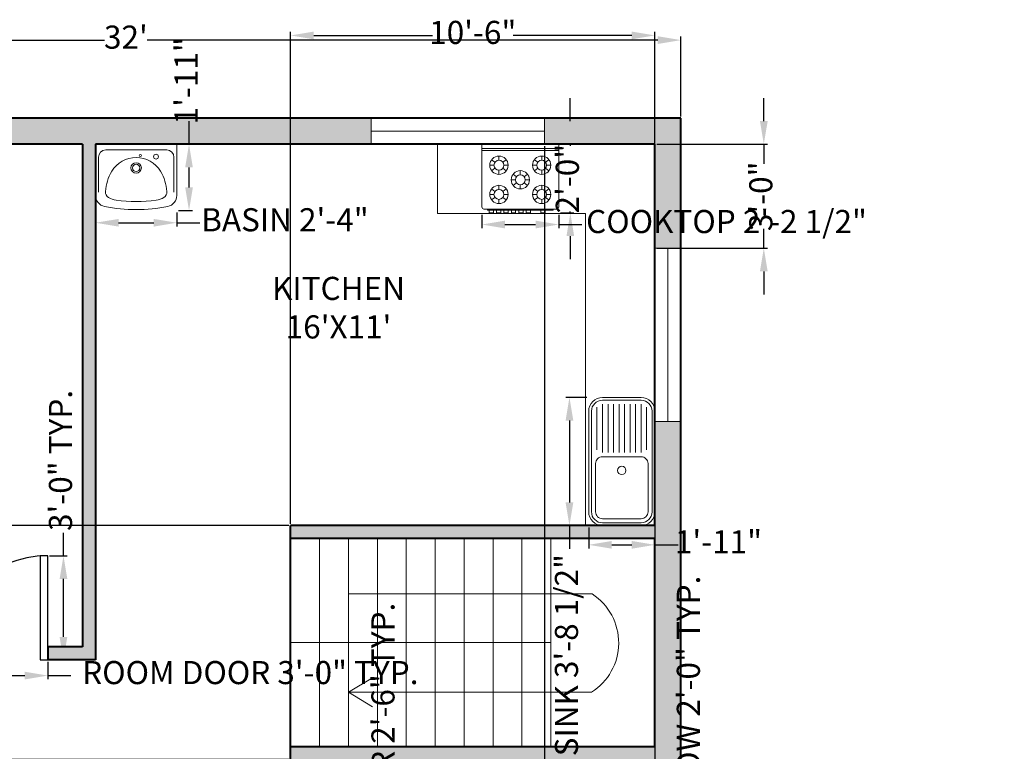
# Model space of a CAD drawing. Units: inches. Extents: x 2138 to 3265, y 2149 to 3392.
# Tile 6 of 13: x 2363 to 2703, y 2511 to 2764. Entities that reach past the tile are written whole.
import ezdxf

# ---------------------------------------------------------------- set-up
doc = ezdxf.new("R2010")
doc.units = ezdxf.units.IN
for name, color, linetype, lineweight in [('A-ANNO-DIMS', 2, 'Continuous', 18), ('A-AREA-IDEN', 7, 'Continuous', 18), ('A-DOOR', 22, 'Continuous', 25), ('A-EQPM', 8, 'Continuous', 18), ('A-FLOR-CASE', 30, 'Continuous', 20), ('A-FLOR-FIXT', 9, 'Continuous', 20), ('A-FLOR-STRS', 7, 'Continuous', 18), ('A-GLAZ', 150, 'Continuous', 18), ('A-WALL', 7, 'Continuous', 40), ('A-WALL-PATT', 142, 'Continuous', 13), ('Washbasin-detail', 251, 'Continuous', 13), ('Washbasin-outline', 250, 'Continuous', 20)]:
    doc.layers.add(name, color=color, linetype=linetype, lineweight=lineweight)
doc.styles.get("Standard").update_dxf_attribs({"font": 'arial.ttf'})
doc.dimstyles.new('ISO-25', dxfattribs={"dimtxt": 8, "dimasz": 8, "dimexe": 1.25, "dimexo": 0.625, "dimtad": 0, "dimdec": 1, "dimlunit": 4, "dimtxsty": 'Standard', "dimcen": 2.5, "dimadec": 0, "dimazin": 0, "dimtfac": 1, "dimtdec": 1, "dimtmove": 0, "dimatfit": 3, "dimfxl": 1, "dimarcsym": 0})

# ---------------------------------------------------------------- blocks, each defined once
blk = doc.blocks.new('g')
for p, q in [((2503.9, 2782.51), (2532.66, 2782.51)), ((2503.9, 2782.51), (2503.9, 2759.08)), ((2532.66, 2782.51), (2532.66, 2759.08)), ((2503.9, 2780.93), (2532.66, 2780.93)), ((2503.9, 2780.15), (2532.66, 2780.15)), ((2508.82, 2775.8), (2507.57, 2776.75)), ((2510.29, 2778.1), (2510.29, 2776.53)), ((2511.76, 2775.8), (2513.02, 2776.75)), ((2524.8, 2775.8), (2523.54, 2776.75)), ((2526.27, 2778.1), (2526.27, 2776.53)), ((2527.74, 2775.8), (2528.99, 2776.75)), ((2508.45, 2774.68), (2506.87, 2774.68)), ((2507.57, 2772.61), (2508.82, 2773.56)), ((2510.29, 2772.83), (2510.29, 2771.26)), ((2513.02, 2772.61), (2511.76, 2773.56)), ((2513.72, 2774.68), (2512.14, 2774.68)), ((2516.81, 2770.34), (2515.56, 2771.29)), ((2518.28, 2772.64), (2518.28, 2771.07)), ((2519.75, 2770.34), (2521.01, 2771.29)), ((2522.85, 2774.68), (2524.42, 2774.68)), ((2523.54, 2772.61), (2524.8, 2773.56)), ((2526.27, 2772.83), (2526.27, 2771.26)), ((2528.99, 2772.61), (2527.74, 2773.56)), ((2528.12, 2774.68), (2529.69, 2774.68)), ((2516.43, 2769.22), (2514.86, 2769.22)), ((2515.56, 2767.15), (2516.81, 2768.1)), ((2521.01, 2767.15), (2519.75, 2768.1)), ((2521.7, 2769.22), (2520.13, 2769.22)), ((2508.45, 2763.75), (2506.87, 2763.75)), ((2507.57, 2765.83), (2508.82, 2764.87)), ((2510.29, 2765.6), (2510.29, 2767.18)), ((2513.02, 2765.83), (2511.76, 2764.87)), ((2513.72, 2763.75), (2512.14, 2763.75)), ((2518.28, 2767.37), (2518.28, 2765.8)), ((2522.85, 2763.75), (2524.42, 2763.75)), ((2523.54, 2765.83), (2524.8, 2764.87)), ((2526.27, 2765.6), (2526.27, 2767.18)), ((2528.99, 2765.83), (2527.74, 2764.87)), ((2528.12, 2763.75), (2529.69, 2763.75)), ((2508.82, 2762.64), (2507.57, 2761.68)), ((2510.29, 2760.33), (2510.29, 2761.91)), ((2511.76, 2762.64), (2513.02, 2761.68)), ((2524.8, 2762.64), (2523.54, 2761.68)), ((2526.27, 2760.33), (2526.27, 2761.91)), ((2527.74, 2762.64), (2528.99, 2761.68)), ((2504.69, 2758.29), (2531.87, 2758.29)), ((2505.99, 2757.9), (2505.99, 2758.29)), ((2505.99, 2757.9), (2530.57, 2757.9)), ((2506.67, 2757.9), (2506.67, 2756.81)), ((2506.67, 2756.81), (2508.27, 2756.81)), ((2508.27, 2756.81), (2508.27, 2757.9)), ((2509.43, 2757.9), (2509.43, 2756.81)), ((2509.43, 2756.81), (2511.02, 2756.81)), ((2511.02, 2756.81), (2511.02, 2757.9)), ((2512.18, 2757.9), (2512.18, 2756.81)), ((2512.18, 2756.81), (2513.78, 2756.81)), ((2513.78, 2756.81), (2513.78, 2757.9)), ((2514.94, 2757.9), (2514.94, 2756.81)), ((2514.94, 2756.81), (2516.54, 2756.81)), ((2516.54, 2756.81), (2516.54, 2757.9)), ((2517.7, 2757.9), (2517.7, 2756.81)), ((2517.7, 2756.81), (2519.29, 2756.81)), ((2519.29, 2756.81), (2519.29, 2757.9)), ((2520.45, 2757.9), (2520.45, 2756.81)), ((2520.45, 2756.81), (2522.05, 2756.81)), ((2522.05, 2756.81), (2522.05, 2757.9)), ((2525.96, 2757.9), (2525.96, 2756.81)), ((2525.96, 2756.81), (2527.56, 2756.81)), ((2527.56, 2756.81), (2527.56, 2757.9)), ((2530.57, 2757.9), (2530.57, 2758.29))]:
    blk.add_line(p, q)
for centre, radius in [((2510.29, 2774.68), 3.42), ((2510.29, 2774.68), 1.85), ((2526.27, 2774.68), 3.42), ((2526.27, 2774.68), 1.85), ((2518.28, 2769.22), 3.42), ((2518.28, 2769.22), 1.85), ((2510.29, 2763.75), 3.42), ((2510.29, 2763.75), 1.85), ((2526.27, 2763.75), 3.42), ((2526.27, 2763.75), 1.85)]:
    blk.add_circle(centre, radius)
for centre, start, end in [((2504.69, 2759.08), 180, 270), ((2531.87, 2759.08), 270, 0)]:
    blk.add_arc(centre, 0.787, start, end)
blk = doc.blocks.new('SINK_KITCHEN_SNGL')
for p, q in [((-39.5, -6), (-8.5, -6)), ((-36.5, -2), (36.5, -2)), ((-44.5, -38), (-44.5, -10)), ((-41.5, -10), (-6.5, -10)), ((-41.5, -14), (-6.5, -14)), ((44.5, -10), (44.5, -38)), ((-41.5, -18), (-6.5, -18)), ((-41.5, -22), (-6.5, -22)), ((-41.5, -26), (-6.5, -26)), ((-41.5, -30), (-6.5, -30)), ((-41.5, -34), (-6.5, -34)), ((-41.5, -38), (-6.5, -38)), ((-39.5, -42), (-8.5, -42)), ((36.5, -46), (-36.5, -46))]:
    blk.add_line(p, q)
at = {"flags": 128}
for points in [[(36.5, 0, -0.414214), (46.5, -10), (46.5, -38, -0.414214), (36.5, -48), (-36.5, -48, -0.414214), (-46.5, -38), (-46.5, -10, -0.414214), (-36.5, 0)], [(36.5, -5, -0.414214), (41.5, -10), (41.5, -38, -0.414214), (36.5, -43), (1.5, -43, -0.414214), (-3.5, -38), (-3.5, -10, -0.414214), (1.5, -5)]]:
    blk.add_lwpolyline(points, format="xyb", close=True, dxfattribs=at)
blk.add_circle((6.5, -24), 3)
for centre, start, end in [((-36.5, -10), 90, 180), ((36.5, -10), 0, 90), ((-36.5, -38), 180, 270), ((36.5, -38), 270, 0)]:
    blk.add_arc(centre, 8, start, end)
blk = doc.blocks.new('sink')
at = {"layer": 'Washbasin-detail'}
for p, q in [((2526.41, 3237.64), (2533.85, 3237.64)), ((2541.29, 3237.64), (2533.85, 3237.64)), ((2524.63, 3235.87), (2524.63, 3227.29)), ((2543.06, 3235.87), (2543.06, 3227.29))]:
    blk.add_line(p, q, dxfattribs=at)
for centre, radius in [((2534.87, 3236.28), 0.263), ((2538.69, 3235.99), 0.591)]:
    blk.add_circle(centre, radius, dxfattribs=at)
for centre, radius, start, end in [((2526.41, 3235.87), 1.77, 90, 180), ((2541.29, 3235.87), 1.77, 0, 90), ((2533.84, 3233.24), 1.28, 90, 270), ((2533.84, 3233.24), 0.886, 90, 270), ((2533.84, 3233.24), 1.28, 270, 90), ((2533.84, 3233.24), 0.886, 270, 90)]:
    blk.add_arc(centre, radius, start, end, dxfattribs=at)
at = {"layer": 'Washbasin-outline'}
for p, q in [((2523.93, 3238.88), (2523.93, 3226.54)), ((2524.06, 3239.02), (2543.63, 3239.02)), ((2543.77, 3238.88), (2543.77, 3226.54))]:
    blk.add_line(p, q, dxfattribs=at)
for centre, radius, start, end in [((2524.06, 3238.88), 0.138, 90, 180), ((2543.63, 3238.88), 0.138, 0, 90), ((2533.85, 3228.86), 6.93, 30.9425, 149.0575), ((2537.35, 3226.75), 11.02, 149.0575, 176.3179), ((2530.34, 3226.75), 11.02, 3.6821, 30.9425), ((2526.68, 3226.54), 2.76, 180, 258.7144), ((2527.93, 3227.36), 1.57, 176.3179, 238.5687), ((2529.57, 3230.05), 4.72, 238.5687, 262.476), ((2533.85, 3262.44), 37.4, 262.476, 277.524), ((2538.13, 3230.05), 4.72, 277.524, 301.4313), ((2539.77, 3227.36), 1.57, 301.4313, 3.6821), ((2541.01, 3226.54), 2.76, 281.2856, 0), ((2533.85, 3262.44), 39.37, 258.7144, 281.2856)]:
    blk.add_arc(centre, radius, start, end, dxfattribs=at)
blk = doc.blocks.new('door')
blk.add_lwpolyline([(2064.92, 2369.1), (2066.69, 2369.1), (2066.69, 2393.11), (2064.92, 2393.11)], close=True)
blk.add_arc((2066.69, 2369.1), 24.02, 90, 180)
blk = doc.blocks.new('*D18')
at = {"layer": 'A-ANNO-DIMS', "color": 0, "lineweight": -2, "transparency": 16777216}
for p, q in [((2207.53, 2730.29), (2207.53, 2757.96)), ((2215.53, 2756.71), (2392.12, 2756.71)), ((2583.53, 2756.71), (2406.94, 2756.71)), ((2591.53, 2730.29), (2591.53, 2757.96))]:
    blk.add_line(p, q, dxfattribs=at)
at = {"layer": 'A-ANNO-DIMS', "color": 0, "transparency": 16777216}
for points in [[(2215.53, 2758.05), (2215.53, 2755.38), (2207.53, 2756.71)], [(2583.53, 2758.05), (2583.53, 2755.38), (2591.53, 2756.71)]]:
    blk.add_solid(points, dxfattribs=at)
at = {"layer": 'Defpoints', "color": 0, "transparency": 16777216}
for p in [(2591.53, 2756.71), (2207.53, 2729.66), (2591.53, 2729.66)]:
    blk.add_point(p, dxfattribs=at)
at = {"layer": 'A-ANNO-DIMS', "color": 0, "transparency": 16777216, "insert": (2399.53, 2756.71), "char_height": 8, "attachment_point": 5}
blk.add_mtext("32'", dxfattribs=at)
blk = doc.blocks.new('GLAZ-SASH-60IN')
for p, q in [((0, 9), (0, 0)), ((60, 9), (60, 0)), ((0, 4.5), (60, 4.5))]:
    blk.add_line(p, q)
blk = doc.blocks.new('*D25')
at = {"layer": 'A-ANNO-DIMS', "color": 0, "lineweight": -2, "transparency": 16777216}
for p, q in [((2595.13, 2443.16), (2595.13, 2451.16)), ((2592.15, 2443.16), (2596.38, 2443.16)), ((2595.13, 2427.16), (2595.13, 2435.16)), ((2592.15, 2419.16), (2596.38, 2419.16))]:
    blk.add_line(p, q, dxfattribs=at)
at = {"layer": 'A-ANNO-DIMS', "color": 0, "transparency": 16777216}
for points in [[(2593.8, 2435.16), (2596.46, 2435.16), (2595.13, 2443.16)], [(2593.8, 2427.16), (2596.46, 2427.16), (2595.13, 2419.16)]]:
    blk.add_solid(points, dxfattribs=at)
at = {"layer": 'Defpoints', "color": 0, "transparency": 16777216}
for p in [(2591.53, 2443.16), (2595.13, 2443.16), (2591.53, 2419.16)]:
    blk.add_point(p, dxfattribs=at)
at = {"layer": 'A-ANNO-DIMS', "color": 0, "transparency": 16777216, "insert": (2595.13, 2513.27), "char_height": 8, "attachment_point": 5, "rotation": 90}
blk.add_mtext('WC WINDOW 2\'-0" TYP.', dxfattribs=at)
blk = doc.blocks.new('*D27')
at = {"layer": 'A-ANNO-DIMS', "color": 0, "lineweight": -2, "transparency": 16777216}
for p, q in [((2336.48, 2541.54), (2336.48, 2535.5)), ((2372.53, 2541.54), (2372.53, 2535.5)), ((2344.48, 2536.75), (2364.53, 2536.75)), ((2372.53, 2536.75), (2380.53, 2536.75))]:
    blk.add_line(p, q, dxfattribs=at)
at = {"layer": 'A-ANNO-DIMS', "color": 0, "transparency": 16777216}
for points in [[(2344.48, 2538.09), (2344.48, 2535.42), (2336.48, 2536.75)], [(2364.53, 2538.09), (2364.53, 2535.42), (2372.53, 2536.75)]]:
    blk.add_solid(points, dxfattribs=at)
at = {"layer": 'Defpoints', "color": 0, "transparency": 16777216}
for p in [(2336.48, 2542.16), (2372.53, 2542.16), (2372.53, 2536.75)]:
    blk.add_point(p, dxfattribs=at)
at = {"layer": 'A-ANNO-DIMS', "color": 0, "transparency": 16777216, "insert": (2442.58, 2536.75), "char_height": 8, "attachment_point": 5}
blk.add_mtext('ROOM DOOR 3\'-0" TYP.', dxfattribs=at)
blk = doc.blocks.new('*D28')
at = {"layer": 'A-ANNO-DIMS', "color": 0, "lineweight": -2, "transparency": 16777216}
for p, q in [((2377.94, 2578.21), (2377.94, 2586.21)), ((2373.15, 2578.21), (2379.19, 2578.21)), ((2377.94, 2550.16), (2377.94, 2570.21)), ((2373.15, 2542.16), (2379.19, 2542.16))]:
    blk.add_line(p, q, dxfattribs=at)
at = {"layer": 'A-ANNO-DIMS', "color": 0, "transparency": 16777216}
for points in [[(2376.6, 2570.21), (2379.27, 2570.21), (2377.94, 2578.21)], [(2376.6, 2550.16), (2379.27, 2550.16), (2377.94, 2542.16)]]:
    blk.add_solid(points, dxfattribs=at)
at = {"layer": 'Defpoints', "color": 0, "transparency": 16777216}
for p in [(2372.53, 2578.21), (2377.94, 2578.21), (2372.53, 2542.16)]:
    blk.add_point(p, dxfattribs=at)
at = {"layer": 'A-ANNO-DIMS', "color": 0, "transparency": 16777216, "insert": (2377.94, 2611.22), "char_height": 8, "attachment_point": 5, "rotation": 90}
blk.add_mtext('3\'-0" TYP.', dxfattribs=at)
blk = doc.blocks.new('*D29')
at = {"layer": 'A-ANNO-DIMS', "color": 0, "lineweight": -2, "transparency": 16777216}
for p, q in [((2489.5, 2449.16), (2489.5, 2457.16)), ((2493.4, 2449.16), (2488.25, 2449.16)), ((2489.5, 2426.94), (2489.5, 2441.16)), ((2493.4, 2418.94), (2488.25, 2418.94))]:
    blk.add_line(p, q, dxfattribs=at)
at = {"layer": 'A-ANNO-DIMS', "color": 0, "transparency": 16777216}
for points in [[(2488.16, 2441.16), (2490.83, 2441.16), (2489.5, 2449.16)], [(2488.16, 2426.94), (2490.83, 2426.94), (2489.5, 2418.94)]]:
    blk.add_solid(points, dxfattribs=at)
at = {"layer": 'Defpoints', "color": 0, "transparency": 16777216}
for p in [(2489.5, 2449.16), (2494.03, 2449.16), (2494.03, 2418.94)]:
    blk.add_point(p, dxfattribs=at)
at = {"layer": 'A-ANNO-DIMS', "color": 0, "transparency": 16777216, "insert": (2489.5, 2511.51), "char_height": 8, "attachment_point": 5, "rotation": 90}
blk.add_mtext('WC DOOR 2\'-6" TYP.', dxfattribs=at)
blk = doc.blocks.new('*D33')
at = {"layer": 'A-ANNO-DIMS', "color": 0, "lineweight": -2, "transparency": 16777216}
for p, q in [((2543.88, 2494.76), (2543.88, 2501.18)), ((2582.53, 2494.76), (2582.53, 2501.18)), ((2551.88, 2499.93), (2574.53, 2499.93)), ((2582.53, 2499.93), (2590.53, 2499.93))]:
    blk.add_line(p, q, dxfattribs=at)
at = {"layer": 'A-ANNO-DIMS', "color": 0, "transparency": 16777216}
for points in [[(2551.88, 2501.26), (2551.88, 2498.6), (2543.88, 2499.93)], [(2574.53, 2501.26), (2574.53, 2498.6), (2582.53, 2499.93)]]:
    blk.add_solid(points, dxfattribs=at)
at = {"layer": 'Defpoints', "color": 0, "transparency": 16777216}
for p in [(2582.53, 2499.93), (2543.88, 2494.13), (2582.53, 2494.13)]:
    blk.add_point(p, dxfattribs=at)
at = {"layer": 'A-ANNO-DIMS', "color": 0, "transparency": 16777216, "insert": (2648.93, 2499.93), "char_height": 8, "attachment_point": 5}
blk.add_mtext('WC PAN 3\'-2 1/2" TYP.', dxfattribs=at)
blk = doc.blocks.new('*D43')
at = {"layer": 'A-ANNO-DIMS', "color": 0, "lineweight": -2, "transparency": 16777216}
for p, q in [((2522.66, 2696.25), (2522.66, 2691.63)), ((2549.28, 2696.25), (2549.28, 2691.63)), ((2530.66, 2692.88), (2541.28, 2692.88)), ((2549.28, 2692.88), (2557.28, 2692.88))]:
    blk.add_line(p, q, dxfattribs=at)
at = {"layer": 'A-ANNO-DIMS', "color": 0, "transparency": 16777216}
for points in [[(2530.66, 2694.22), (2530.66, 2691.55), (2522.66, 2692.88)], [(2541.28, 2694.22), (2541.28, 2691.55), (2549.28, 2692.88)]]:
    blk.add_solid(points, dxfattribs=at)
at = {"layer": 'Defpoints', "color": 0, "transparency": 16777216}
for p in [(2522.66, 2696.88), (2549.28, 2696.88), (2549.28, 2692.88)]:
    blk.add_point(p, dxfattribs=at)
at = {"layer": 'A-ANNO-DIMS', "color": 0, "transparency": 16777216, "insert": (2607.31, 2692.88), "char_height": 8, "attachment_point": 5}
blk.add_mtext('COOKTOP 2\'-2 1/2"', dxfattribs=at)
blk = doc.blocks.new('*D44')
at = {"layer": 'A-ANNO-DIMS', "color": 0, "lineweight": -2, "transparency": 16777216}
for p, q in [((2553.27, 2728.66), (2553.27, 2736.66)), ((2549.9, 2720.66), (2554.52, 2720.66)), ((2553.27, 2720.66), (2553.27, 2720.1)), ((2549.9, 2696.88), (2554.52, 2696.88)), ((2553.27, 2696.88), (2553.27, 2697.44)), ((2553.27, 2688.88), (2553.27, 2680.88))]:
    blk.add_line(p, q, dxfattribs=at)
at = {"layer": 'A-ANNO-DIMS', "color": 0, "transparency": 16777216}
for points in [[(2551.94, 2728.66), (2554.6, 2728.66), (2553.27, 2720.66)], [(2551.94, 2688.88), (2554.6, 2688.88), (2553.27, 2696.88)]]:
    blk.add_solid(points, dxfattribs=at)
at = {"layer": 'Defpoints', "color": 0, "transparency": 16777216}
for p in [(2549.28, 2720.66), (2553.27, 2720.66), (2549.28, 2696.88)]:
    blk.add_point(p, dxfattribs=at)
at = {"layer": 'A-ANNO-DIMS', "color": 0, "transparency": 16777216, "insert": (2553.27, 2708.77), "char_height": 8, "attachment_point": 5, "rotation": 90}
blk.add_mtext('2\'-0"', dxfattribs=at)
blk = doc.blocks.new('*D45')
at = {"layer": 'A-ANNO-DIMS', "color": 0, "lineweight": -2, "transparency": 16777216}
for p, q in [((2559, 2633.03), (2551.72, 2633.03)), ((2552.97, 2625.03), (2552.97, 2596.66)), ((2559, 2588.66), (2551.72, 2588.66)), ((2552.97, 2588.66), (2552.97, 2580.66))]:
    blk.add_line(p, q, dxfattribs=at)
at = {"layer": 'A-ANNO-DIMS', "color": 0, "transparency": 16777216}
for points in [[(2551.64, 2625.03), (2554.31, 2625.03), (2552.97, 2633.03)], [(2551.64, 2596.66), (2554.31, 2596.66), (2552.97, 2588.66)]]:
    blk.add_solid(points, dxfattribs=at)
at = {"layer": 'Defpoints', "color": 0, "transparency": 16777216}
for p in [(2559.63, 2633.03), (2552.97, 2588.66), (2559.63, 2588.66)]:
    blk.add_point(p, dxfattribs=at)
at = {"layer": 'A-ANNO-DIMS', "color": 0, "transparency": 16777216, "insert": (2552.97, 2519.59), "char_height": 8, "attachment_point": 5, "rotation": 90}
blk.add_mtext('KITCHEN SINK 3\'-8 1/2"', dxfattribs=at)
blk = doc.blocks.new('*D46')
at = {"layer": 'A-ANNO-DIMS', "color": 0, "lineweight": -2, "transparency": 16777216}
for p, q in [((2559.63, 2588.04), (2559.63, 2580.76)), ((2582.53, 2588.04), (2582.53, 2580.76)), ((2567.63, 2582.01), (2574.53, 2582.01)), ((2582.53, 2582.01), (2590.53, 2582.01))]:
    blk.add_line(p, q, dxfattribs=at)
at = {"layer": 'A-ANNO-DIMS', "color": 0, "transparency": 16777216}
for points in [[(2567.63, 2583.34), (2567.63, 2580.67), (2559.63, 2582.01)], [(2574.53, 2583.34), (2574.53, 2580.67), (2582.53, 2582.01)]]:
    blk.add_solid(points, dxfattribs=at)
at = {"layer": 'Defpoints', "color": 0, "transparency": 16777216}
for p in [(2559.63, 2588.66), (2582.53, 2588.66), (2582.53, 2582.01)]:
    blk.add_point(p, dxfattribs=at)
at = {"layer": 'A-ANNO-DIMS', "color": 0, "transparency": 16777216, "insert": (2604.52, 2582.01), "char_height": 8, "attachment_point": 5}
blk.add_mtext('1\'-11"', dxfattribs=at)
blk = doc.blocks.new('*D47')
at = {"layer": 'A-ANNO-DIMS', "color": 0, "lineweight": -2, "transparency": 16777216}
for p, q in [((2389.03, 2697.08), (2389.03, 2692.24)), ((2417.15, 2697.08), (2417.15, 2692.24)), ((2397.03, 2693.49), (2409.15, 2693.49)), ((2417.15, 2693.49), (2425.15, 2693.49))]:
    blk.add_line(p, q, dxfattribs=at)
at = {"layer": 'A-ANNO-DIMS', "color": 0, "transparency": 16777216}
for points in [[(2397.03, 2694.82), (2397.03, 2692.15), (2389.03, 2693.49)], [(2409.15, 2694.82), (2409.15, 2692.15), (2417.15, 2693.49)]]:
    blk.add_solid(points, dxfattribs=at)
at = {"layer": 'Defpoints', "color": 0, "transparency": 16777216}
for p in [(2389.03, 2697.7), (2417.15, 2697.7), (2417.15, 2693.49)]:
    blk.add_point(p, dxfattribs=at)
at = {"layer": 'A-ANNO-DIMS', "color": 0, "transparency": 16777216, "insert": (2454.55, 2693.49), "char_height": 8, "attachment_point": 5}
blk.add_mtext('BASIN 2\'-4"', dxfattribs=at)
blk = doc.blocks.new('*D48')
at = {"layer": 'A-ANNO-DIMS', "color": 0, "lineweight": -2, "transparency": 16777216}
for p, q in [((2421.37, 2720.66), (2421.37, 2728.66)), ((2417.78, 2720.66), (2422.62, 2720.66)), ((2421.37, 2705.7), (2421.37, 2712.66)), ((2417.78, 2697.7), (2422.62, 2697.7))]:
    blk.add_line(p, q, dxfattribs=at)
at = {"layer": 'A-ANNO-DIMS', "color": 0, "transparency": 16777216}
for points in [[(2420.04, 2712.66), (2422.7, 2712.66), (2421.37, 2720.66)], [(2420.04, 2705.7), (2422.7, 2705.7), (2421.37, 2697.7)]]:
    blk.add_solid(points, dxfattribs=at)
at = {"layer": 'Defpoints', "color": 0, "transparency": 16777216}
for p in [(2417.15, 2720.66), (2421.37, 2720.66), (2417.15, 2697.7)]:
    blk.add_point(p, dxfattribs=at)
at = {"layer": 'A-ANNO-DIMS', "color": 0, "transparency": 16777216, "insert": (2421.37, 2742.65), "char_height": 8, "attachment_point": 5, "rotation": 90}
blk.add_mtext('1\'-11"', dxfattribs=at)
blk = doc.blocks.new('*D54')
at = {"layer": 'A-ANNO-DIMS', "color": 0, "lineweight": -2, "transparency": 16777216}
for p, q in [((2456.53, 2589.29), (2456.53, 2759.59)), ((2582.53, 2589.29), (2582.53, 2759.59)), ((2464.53, 2758.34), (2505.54, 2758.34)), ((2574.53, 2758.34), (2533.52, 2758.34))]:
    blk.add_line(p, q, dxfattribs=at)
at = {"layer": 'A-ANNO-DIMS', "color": 0, "transparency": 16777216}
for points in [[(2464.53, 2759.67), (2464.53, 2757), (2456.53, 2758.34)], [(2574.53, 2759.67), (2574.53, 2757), (2582.53, 2758.34)]]:
    blk.add_solid(points, dxfattribs=at)
at = {"layer": 'Defpoints', "color": 0, "transparency": 16777216}
for p in [(2582.53, 2758.34), (2456.53, 2588.66), (2582.53, 2588.66)]:
    blk.add_point(p, dxfattribs=at)
at = {"layer": 'A-ANNO-DIMS', "color": 0, "transparency": 16777216, "insert": (2519.53, 2758.34), "char_height": 8, "attachment_point": 5}
blk.add_mtext('10\'-6"', dxfattribs=at)
blk = doc.blocks.new('*D55')
at = {"layer": 'A-ANNO-DIMS', "color": 0, "lineweight": -2, "transparency": 16777216}
for p, q in [((2455.9, 2588.66), (2177.6, 2588.66)), ((2178.85, 2580.66), (2178.85, 2559.44)), ((2178.85, 2515.66), (2178.85, 2536.88)), ((2455.9, 2507.66), (2177.6, 2507.66))]:
    blk.add_line(p, q, dxfattribs=at)
at = {"layer": 'A-ANNO-DIMS', "color": 0, "transparency": 16777216}
for points in [[(2177.52, 2580.66), (2180.19, 2580.66), (2178.85, 2588.66)], [(2177.52, 2515.66), (2180.19, 2515.66), (2178.85, 2507.66)]]:
    blk.add_solid(points, dxfattribs=at)
at = {"layer": 'Defpoints', "color": 0, "transparency": 16777216}
for p in [(2456.53, 2588.66), (2178.85, 2507.66), (2456.53, 2507.66)]:
    blk.add_point(p, dxfattribs=at)
at = {"layer": 'A-ANNO-DIMS', "color": 0, "transparency": 16777216, "insert": (2178.85, 2548.16), "char_height": 8, "attachment_point": 5, "rotation": 90}
blk.add_mtext('6\'-9"', dxfattribs=at)
blk = doc.blocks.new('*D57')
at = {"layer": 'A-ANNO-DIMS', "color": 0, "lineweight": -2, "transparency": 16777216}
for p, q in [((2620.2, 2728.66), (2620.2, 2736.66)), ((2583.15, 2720.66), (2621.45, 2720.66)), ((2620.2, 2720.66), (2620.2, 2713.92)), ((2620.2, 2684.66), (2620.2, 2691.41)), ((2583.15, 2684.66), (2621.45, 2684.66)), ((2620.2, 2676.66), (2620.2, 2668.66))]:
    blk.add_line(p, q, dxfattribs=at)
at = {"layer": 'A-ANNO-DIMS', "color": 0, "transparency": 16777216}
for points in [[(2618.87, 2728.66), (2621.54, 2728.66), (2620.2, 2720.66)], [(2618.87, 2676.66), (2621.54, 2676.66), (2620.2, 2684.66)]]:
    blk.add_solid(points, dxfattribs=at)
at = {"layer": 'Defpoints', "color": 0, "transparency": 16777216}
for p in [(2582.53, 2720.66), (2582.53, 2684.66), (2620.2, 2684.66)]:
    blk.add_point(p, dxfattribs=at)
at = {"layer": 'A-ANNO-DIMS', "color": 0, "transparency": 16777216, "insert": (2620.2, 2702.66), "char_height": 8, "attachment_point": 5, "rotation": 90}
blk.add_mtext('3\'-0"', dxfattribs=at)
blk = doc.blocks.new('*D58')
at = {"layer": 'A-ANNO-DIMS', "color": 0, "lineweight": -2, "transparency": 16777216}
for p, q in [((2544.36, 2720.04), (2544.36, 2159.74)), ((2582.53, 2720.04), (2582.53, 2159.74)), ((2536.36, 2160.99), (2528.36, 2160.99)), ((2544.36, 2160.99), (2552.19, 2160.99)), ((2582.53, 2160.99), (2574.7, 2160.99)), ((2590.53, 2160.99), (2598.53, 2160.99))]:
    blk.add_line(p, q, dxfattribs=at)
at = {"layer": 'A-ANNO-DIMS', "color": 0, "transparency": 16777216}
for points in [[(2536.36, 2162.32), (2536.36, 2159.65), (2544.36, 2160.99)], [(2590.53, 2162.32), (2590.53, 2159.65), (2582.53, 2160.99)]]:
    blk.add_solid(points, dxfattribs=at)
at = {"layer": 'Defpoints', "color": 0, "transparency": 16777216}
for p in [(2544.36, 2720.66), (2582.53, 2720.66), (2544.36, 2160.99)]:
    blk.add_point(p, dxfattribs=at)
at = {"layer": 'A-ANNO-DIMS', "color": 0, "transparency": 16777216, "insert": (2563.45, 2160.99), "char_height": 8, "attachment_point": 5}
blk.add_mtext('3\'-2"', dxfattribs=at)

msp = doc.modelspace()

# ---------------------------------------------------------------- hatches: boundary and pattern name
at = {"layer": 'A-WALL-PATT'}
h = msp.add_hatch(color=256, dxfattribs=at)
h.dxf.hatch_style = 1
h.paths.add_polyline_path([(2270.53, 2729.66), (2207.53, 2729.66), (2207.53, 2663.66), (2216.53, 2663.66), (2216.53, 2720.66), (2270.53, 2720.66)])
h.paths.add_polyline_path([(2484.36, 2729.66), (2330.53, 2729.66), (2330.53, 2720.66), (2384.53, 2720.66), (2384.53, 2546.66), (2372.53, 2546.66), (2372.53, 2542.16), (2389.03, 2542.16), (2389.03, 2720.66), (2484.36, 2720.66)])
h.paths.add_polyline_path([(2591.53, 2729.66), (2544.36, 2729.66), (2544.36, 2720.66), (2582.53, 2720.66), (2582.53, 2684.66), (2591.53, 2684.66)])
h.paths.add_polyline_path([(2591.53, 2624.66), (2582.53, 2624.66), (2582.53, 2588.66), (2456.53, 2588.66), (2456.53, 2584.16), (2582.53, 2584.16), (2582.53, 2512.16), (2456.53, 2512.16), (2456.53, 2507.66), (2494.03, 2507.66), (2494.03, 2501.66), (2498.53, 2501.66), (2498.53, 2507.66), (2582.53, 2507.66), (2582.53, 2495.66), (2591.53, 2495.66)])
h.paths.add_polyline_path([(2591.53, 2471.66), (2582.53, 2471.66), (2582.53, 2459.66), (2498.53, 2459.66), (2498.53, 2471.66), (2497.72, 2471.66, -0.030629), (2494.03, 2471.44), (2494.03, 2459.66), (2431.08, 2459.66, -0.013128), (2431.03, 2457.77), (2431.03, 2455.16), (2494.03, 2455.16), (2494.03, 2449.16), (2498.53, 2449.16), (2498.53, 2455.16), (2582.53, 2455.16), (2582.53, 2443.16), (2591.53, 2443.16)])
h.paths.add_polyline_path([(2591.53, 2419.16), (2582.53, 2419.16), (2582.53, 2407.16), (2498.53, 2407.16), (2498.53, 2419.16), (2497.72, 2419.16, -0.030629), (2494.03, 2418.94), (2494.03, 2402.66), (2582.53, 2402.66), (2582.53, 2360.66), (2591.53, 2360.66)])
h.paths.add_polyline_path([(2591.53, 2300.66), (2582.53, 2300.66), (2582.53, 2258.66), (2515.78, 2258.66), (2515.78, 2249.66), (2591.53, 2249.66)])
h.paths.add_polyline_path([(2455.78, 2258.66), (2389.03, 2258.66), (2389.03, 2455.16), (2395.03, 2455.16), (2395.03, 2459.66), (2384.53, 2459.66), (2384.53, 2258.66), (2375.53, 2258.66), (2375.53, 2249.66), (2455.78, 2249.66)])
h.paths.add_polyline_path([(2315.53, 2253.24), (2315.53, 2258.66), (2296.03, 2258.66), (2296.03, 2249.66), (2315.53, 2249.66)])
h.paths.add_polyline_path([(2236.03, 2258.66), (2216.53, 2258.66), (2216.53, 2290.16), (2207.53, 2290.16), (2207.53, 2249.66), (2236.03, 2249.66)])
h.paths.add_polyline_path([(2216.53, 2396.66), (2207.53, 2396.66), (2207.53, 2350.16), (2216.53, 2350.16)])
h.paths.add_polyline_path([(2216.53, 2603.66), (2207.53, 2603.66), (2207.53, 2456.66), (2216.53, 2456.66), (2216.53, 2542.16), (2264.53, 2542.16), (2264.53, 2470.16), (2252.53, 2470.16), (2252.53, 2465.66), (2269.03, 2465.66), (2269.03, 2542.16), (2336.48, 2542.16, -0.013128), (2336.53, 2544.05), (2336.53, 2546.66), (2216.53, 2546.66)])

# ---------------------------------------------------------------- linework, layer by layer
at = {"layer": 'A-FLOR-CASE'}
for p, q in [((2507.33, 2720.66), (2507.33, 2696.66)), ((2558.53, 2696.66), (2507.33, 2696.66)), ((2558.53, 2588.66), (2558.53, 2696.66))]:
    msp.add_line(p, q, dxfattribs=at)
at = {"layer": 'A-FLOR-STRS'}
for p, q in [((2466.53, 2512.16), (2466.53, 2584.16)), ((2476.53, 2512.16), (2476.53, 2584.16)), ((2486.53, 2512.16), (2486.53, 2584.16)), ((2496.53, 2512.16), (2496.53, 2584.16)), ((2506.53, 2512.16), (2506.53, 2584.16)), ((2516.53, 2512.16), (2516.53, 2584.16)), ((2526.53, 2512.16), (2526.53, 2584.16)), ((2536.53, 2512.16), (2536.53, 2584.16)), ((2546.53, 2512.16), (2546.53, 2584.16)), ((2476.53, 2564.99), (2560.81, 2564.99)), ((2546.53, 2548.16), (2456.53, 2548.16)), ((2476.53, 2530.96), (2484.84, 2536.02)), ((2476.53, 2530.96), (2560.55, 2530.96)), ((2476.53, 2530.96), (2484.84, 2525.91))]:
    msp.add_line(p, q, dxfattribs=at)
msp.add_arc((2549.82, 2548.06), 20.19, 302.1215, 57.0071, dxfattribs=at)
at = {"layer": 'A-GLAZ'}
for p, q in [((2544.36, 2720.66), (2544.36, 2729.66)), ((2484.36, 2725.16), (2544.36, 2725.16))]:
    msp.add_line(p, q, dxfattribs=at)
for points in [[(2484.36, 2729.66), (2544.36, 2729.66), (2544.36, 2720.66), (2484.36, 2720.66)], [(2582.53, 2684.66), (2591.53, 2684.66), (2591.53, 2624.66), (2582.53, 2624.66)]]:
    msp.add_lwpolyline(points, close=True, dxfattribs=at)
at = {"layer": 'A-WALL'}
for p, q in [((2591.53, 2729.66), (2207.53, 2729.66)), ((2591.53, 2249.66), (2591.53, 2729.66)), ((2384.53, 2720.66), (2216.53, 2720.66)), ((2384.53, 2720.66), (2384.53, 2546.66)), ((2582.53, 2720.66), (2389.03, 2720.66)), ((2389.03, 2720.66), (2389.03, 2542.16)), ((2582.53, 2588.66), (2582.53, 2720.66)), ((2582.53, 2588.66), (2456.53, 2588.66)), ((2456.53, 2507.66), (2456.53, 2588.66)), ((2582.53, 2584.16), (2456.53, 2584.16)), ((2582.53, 2512.16), (2582.53, 2584.16)), ((2384.53, 2546.66), (2372.53, 2546.66)), ((2372.53, 2546.66), (2372.53, 2542.16)), ((2389.03, 2542.16), (2372.53, 2542.16)), ((2456.53, 2512.16), (2582.53, 2512.16))]:
    msp.add_line(p, q, dxfattribs=at)

# ---------------------------------------------------------------- block references
at = {"layer": 'A-DOOR', "xscale": 1.501085369916538, "yscale": 1.501085369916538, "zscale": 1.501085369916538}
msp.add_blockref('door', (-729.75, -1014.05), dxfattribs=at)
at = {"layer": 'A-EQPM', "xscale": 0.9255248790432627, "yscale": 0.9255248790432627, "zscale": 0.9255248790432627}
msp.add_blockref('g', (205.24, 145.38), dxfattribs=at)
at = {"layer": 'A-FLOR-FIXT', "xscale": 1.417224490882656, "yscale": 1.417224490882656, "zscale": 1.417224490882656}
msp.add_blockref('sink', (-1187.94, -1869.76), dxfattribs=at)
at = {"layer": 'A-FLOR-FIXT', "xscale": 0.4771174957545016, "yscale": 0.4771174957545016, "zscale": 0.4771174957545016, "rotation": 270}
msp.add_blockref('SINK_KITCHEN_SNGL', (2582.53, 2610.85), dxfattribs=at)
at = {"layer": 'A-GLAZ', "rotation": 89.99999999999916}
msp.add_blockref('GLAZ-SASH-60IN', (2591.53, 2624.66), dxfattribs=at)

# ---------------------------------------------------------------- texts
at = {"layer": 'A-AREA-IDEN', "insert": (2434.58, 2674.77), "char_height": 8, "attachment_point": 1}
msp.add_mtext_dynamic_manual_height_columns("\\pxqc;KITCHEN\\P16'X11'", width=77.0226, gutter_width=12.5, heights=[0], dxfattribs=at)

# ---------------------------------------------------------------- dimensions: what is measured, and where the dimension line sits
at = {"layer": 'A-ANNO-DIMS'}
for base, p1, p2, override, picture, middle in [((2582.53, 2758.34), (2456.53, 2588.66), (2582.53, 2588.66), {"dimdec": 1, "dimlfac": 1, "dimrnd": 0, "dimzin": 1, "dimdsep": 46, "dimlunit": 4, "dimfrac": 2}, '*D54', (2519.53, 2758.34)), ((2591.53, 2756.71), (2207.53, 2729.66), (2591.53, 2729.66), {"dimclrd": 0, "dimclre": 0, "dimclrt": 0}, '*D18', (2399.53, 2756.71)), ((2544.36, 2160.99), (2582.53, 2720.66), (2544.36, 2720.66), {"dimdec": 1, "dimlfac": 1, "dimrnd": 0, "dimzin": 1, "dimdsep": 46, "dimlunit": 4, "dimfrac": 2}, '*D58', (2563.45, 2160.99)), ((2582.53, 2582.01), (2559.63, 2588.66), (2582.53, 2588.66), {"dimdec": 1, "dimlfac": 1, "dimrnd": 0, "dimzin": 1, "dimdsep": 46, "dimlunit": 4, "dimfrac": 2}, '*D46', (2604.52, 2582.01))]:
    dim = msp.add_linear_dim(base=base, p1=p1, p2=p2, dimstyle='ISO-25', override=override, dxfattribs=at)
    dim.commit()
    dim.dimension.update_dxf_attribs({"geometry": picture, "text_midpoint": middle})
for base, p1, p2, picture, middle in [((2421.37, 2720.66), (2417.15, 2697.7), (2417.15, 2720.66), '*D48', (2421.37, 2742.65)), ((2553.27, 2720.66), (2549.28, 2696.88), (2549.28, 2720.66), '*D44', (2553.27, 2708.77)), ((2620.2, 2684.66), (2582.53, 2720.66), (2582.53, 2684.66), '*D57', (2620.2, 2702.66)), ((2178.85, 2507.66), (2456.53, 2588.66), (2456.53, 2507.66), '*D55', (2178.85, 2548.16))]:
    dim = msp.add_linear_dim(base=base, p1=p1, p2=p2, angle=90, dimstyle='ISO-25', override={"dimdec": 1, "dimlfac": 1, "dimrnd": 0, "dimzin": 1, "dimdsep": 46, "dimlunit": 4, "dimfrac": 2}, dxfattribs=at)
    dim.commit()
    dim.dimension.update_dxf_attribs({"geometry": picture, "text_midpoint": middle})
for base, p1, p2, text, picture, middle in [((2549.28, 2692.88), (2522.66, 2696.88), (2549.28, 2696.88), 'COOKTOP <>', '*D43', (2607.31, 2692.88)), ((2417.15, 2693.49), (2389.03, 2697.7), (2417.15, 2697.7), 'BASIN <>', '*D47', (2454.55, 2693.49)), ((2372.5295, 2536.7541), (2336.4798, 2542.1616), (2372.5295, 2542.1616), 'ROOM DOOR <> TYP.', '*D27', (2442.5815, 2536.7541)), ((2582.5295, 2499.9306), (2543.8826, 2494.1336), (2582.5295, 2494.1336), 'WC PAN <> TYP.', '*D33', (2648.9253, 2499.9306))]:
    dim = msp.add_linear_dim(base=base, p1=p1, p2=p2, text=text, dimstyle='ISO-25', override={"dimdec": 1, "dimlfac": 1, "dimrnd": 0, "dimzin": 1, "dimdsep": 46, "dimlunit": 4, "dimfrac": 2}, dxfattribs=at)
    dim.commit()
    dim.dimension.update_dxf_attribs({"geometry": picture, "text_midpoint": middle})
for base, p1, p2, angle, text, picture, middle in [((2377.937, 2578.2113), (2372.5295, 2542.1616), (2372.5295, 2578.2113), 90, '<> TYP.', '*D28', (2377.937, 2611.2155)), ((2552.97, 2588.66), (2559.63, 2633.03), (2559.63, 2588.66), 270, 'KITCHEN SINK <>', '*D45', (2552.97, 2519.59)), ((2595.13, 2443.16), (2591.53, 2419.16), (2591.53, 2443.16), 90, 'WC WINDOW <> TYP.', '*D25', (2595.13, 2513.27)), ((2489.5, 2449.16), (2494.03, 2418.94), (2494.03, 2449.16), 90, 'WC DOOR <> TYP.', '*D29', (2489.5, 2511.51))]:
    dim = msp.add_linear_dim(base=base, p1=p1, p2=p2, angle=angle, text=text, dimstyle='ISO-25', override={"dimdec": 1, "dimlfac": 1, "dimrnd": 0, "dimzin": 1, "dimdsep": 46, "dimlunit": 4, "dimfrac": 2}, dxfattribs=at)
    dim.commit()
    dim.dimension.update_dxf_attribs({"geometry": picture, "text_midpoint": middle})

doc.saveas('drawing.dxf')
